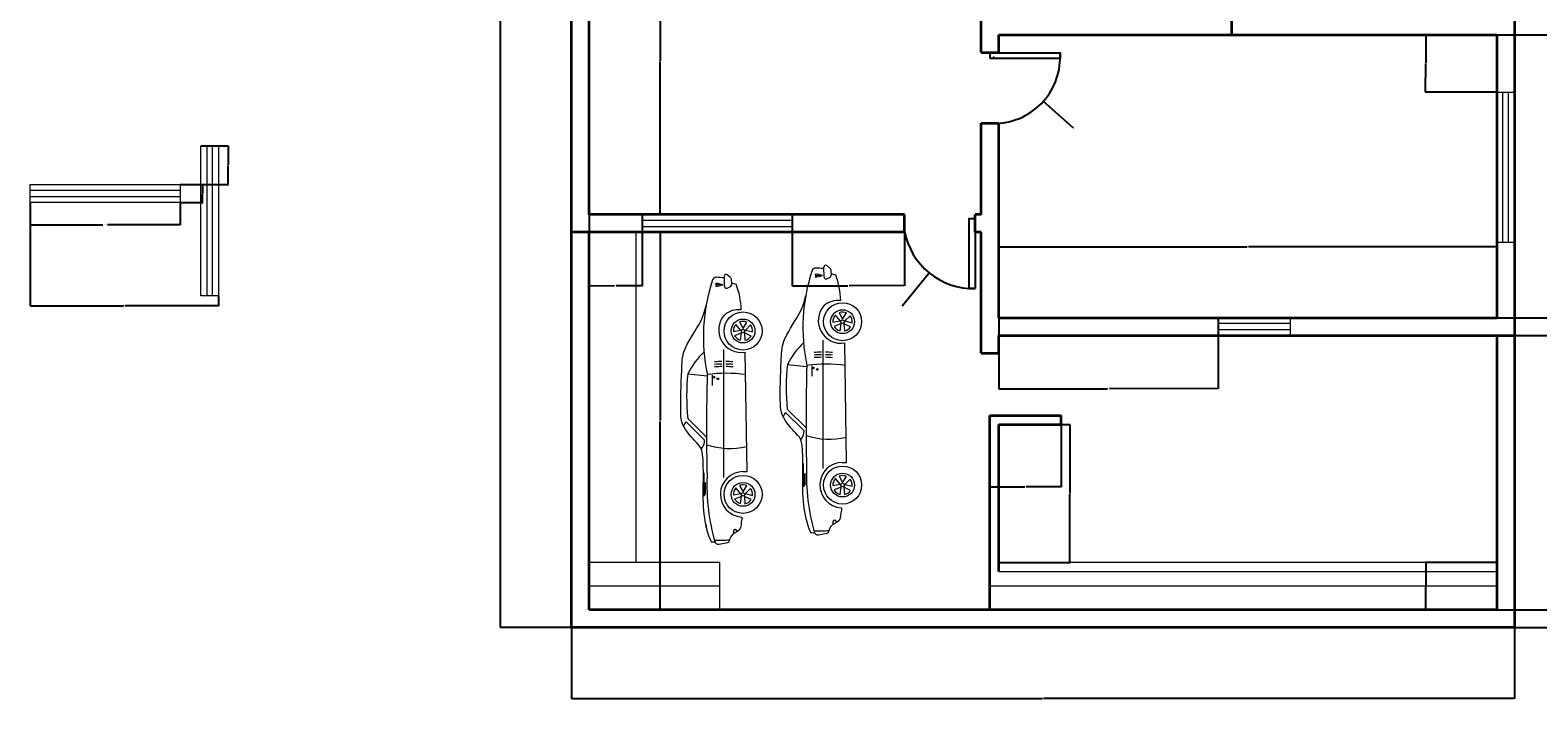
# Model space of a CAD drawing. Units: inches. Extents: x -52 to 1967, y 32 to 824.
# Tile 1 of 10: x -52 to 715, y 32 to 372. Entities that reach past the tile are written whole.
import ezdxf

# ---------------------------------------------------------------- set-up
doc = ezdxf.new("R2010")
doc.units = ezdxf.units.IN
for name, color, linetype, lineweight in [('A-ANNO-DIMS', 2, 'Continuous', 18), ('A-DOOR', 3, 'Continuous', 25), ('A-FLOR', 7, 'Continuous', 18), ('A-GLAZ', 4, 'Continuous', 18), ('A-SITE-VEHI', 8, 'Continuous', 13), ('A-WALL', 7, 'Continuous', 35)]:
    doc.layers.add(name, color=color, linetype=linetype, lineweight=lineweight)
doc.styles.get("Standard").update_dxf_attribs({"font": 'arial.ttf'})
doc.dimstyles.get("Standard").update_dxf_attribs({"dimtxt": 0.18, "dimasz": 0.18, "dimexe": 0.18, "dimexo": 0.0625, "dimgap": 0.09, "dimtad": 0, "dimtih": 1, "dimtoh": 1, "dimdec": 4, "dimzin": 0, "dimdsep": 46, "dimtxsty": 'Standard', "dimcen": 0.09, "dimadec": 0, "dimazin": 0, "dimtfac": 1, "dimtdec": 4, "dimtofl": 0, "dimtmove": 0, "dimatfit": 3, "dimfxl": 1, "dimtolj": 1, "dimtzin": 0, "dimarcsym": 0})

# ---------------------------------------------------------------- blocks, each defined once
blk = doc.blocks.new('*U16')
for p, q in [((72.9, 40.2), (85.8, 53.2)), ((75, 38.8), (88.1, 52)), ((119.4, 51.9), (117.9, 38.3)), ((50.1, 41.1), (34.3, 41)), ((43.3, 39.8), (35.2, 39.8)), ((35.3, 40.5), (50.1, 40.6)), ((111.1, 34.7), (118.5, 34.6)), ((46.7, 26.8), (136.3, 26.8)), ((179.3, 24.4), (180.3, 22.5)), ((180.4, 26.2), (187.5, 26.4)), ((182.6, 21.1), (184.9, 21.3)), ((186.7, 22.2), (188.5, 24.4)), ((7.4, 19.8), (9.7, 19.8)), ((9.8, 17.9), (8.5, 17.9)), ((10.4, 19.2), (10.4, 18.6)), ((50.9, 13.5), (50.9, 10.5))]:
    blk.add_line(p, q)
for points in [[(35.3, 39.9), (35.3, 40.3, 0.269532), (35.1, 40.5), (34.4, 41, 0.575383), (34.2, 40.8), (34.2, 40.5, 0.269532), (34.3, 40.2), (35.1, 39.8, 0.575383)], [(31.3, 7.7), (33.5, 12.4), (28.4, 12, 0.199906)], [(28.5, 15.1), (33.6, 14.4), (31.7, 19.2, 0.199906)], [(39.2, 8.1), (35.5, 11.7), (34.2, 6.7, 0.199906)], [(34.6, 20.1), (35.6, 15), (39.5, 18.3, 0.199906)], [(41.2, 15.7), (36.7, 13.3), (41.1, 10.6, 0.199906)], [(142.8, 15.1), (148, 14.4), (146, 19.2, 0.199906)], [(145.7, 7.7), (147.9, 12.4), (142.8, 12, 0.199906)], [(153.5, 8.1), (149.8, 11.7), (148.6, 6.7, 0.199906)], [(149, 20.1), (149.9, 15), (153.9, 18.3, 0.199906)], [(155.6, 15.7), (151.1, 13.3), (155.4, 10.6, 0.199906)]]:
    blk.add_lwpolyline(points, format="xyb", close=True)
for points in [[(181.6, 27.5), (181.5, 31.9), (180.5, 32.4)], [(181.6, 27.5), (181.5, 31.9), (182.6, 32.5)], [(50.9, 10.5), (134.4, 11.8)]]:
    blk.add_lwpolyline(points)
for centre, radius in [((35, 13.3), 13.3), ((35, 13.3), 8.35), ((115.9, 31), 0.619), ((149.3, 13.3), 13.3), ((149.3, 13.3), 8.35), ((35, 13.3), 1.25), ((149.3, 13.3), 1.25)]:
    blk.add_circle(centre, radius)
for centre, radius, start, end in [((114.6, 105.1), 59.4, 237.6103, 240.9785), ((103.5, -95), 147.8, 83.8163, 95.9705), ((73.3, 50.5), 10.3, 230.424, 268.0085), ((95.5, 3.9), 53.6, 43.2748, 63.5665), ((42.2, -111.3), 149.9, 87.8393, 105.8096), ((20.5, -3.2), 43.1, 98.5304, 116.112), ((79.2, 30.1), 76.3, 177.5773, 185.5205), ((80.1, -1364.1), 1403, 88.423, 91.3179), ((118.3, 22.5), 51.2, 161.4307, 193.2363), ((145.2, -84.9), 126, 71.5283, 102.1242), ((25.7, 24.9), 94, 351.8279, 8.1674), ((45.6, 26.8), 78.8, 0.852, 4.6556), ((47.4, 26.9), 78.8, 0.852, 4.6556), ((49.2, 26.9), 78.8, 0.852, 4.6556), ((216.3, 37.8), 36.2, 188.4683, 196.5315), ((146.7, 37), 36.2, 344.7432, 352.8063), ((184.3, 32.3), 2.49, 357.932, 71.5283), ((116.6, 34.7), 70.3, 353.1942, 357.932), ((35, 13.3), 15.9, 0.6373, 176.3412), ((45.6, 26.8), 78.8, 355.2644, 358.8633), ((47.4, 26.9), 78.8, 355.2644, 358.8633), ((49.2, 26.9), 78.8, 355.2644, 358.8633), ((150.1, 14.4), 15.9, 49.2263, 189.1528), ((149.4, 16.5), 14.8, 352.7285, 41.6613), ((180.4, 24.9), 1.25, 91.939, 207.109), ((182.5, 23.6), 2.49, 207.109, 273.4677), ((114.2, 37), 70.3, 344.3985, 346.9385), ((184.8, 23.8), 2.49, 273.4677, 320.1683), ((187.6, 25.2), 1.25, 320.1683, 91.939), ((9.7, 19.2), 0.623, 0.6373, 90.6373), ((9.8, 18.6), 0.623, 270.6373, 0.6373), ((162.5, 70.8), 56.2, 271.6865, 290.2774)]:
    blk.add_arc(centre, radius, start, end)
blk.add_ellipse((116.9, 33.6), major_axis=(-0.63, -0.007), ratio=0.610043)
for points, knots in [([(11.4, 38.9), (18.1, 40.2), (30.9, 42), (64.8, 40.1), (70.2, 44.9), (82.4, 56.4), (99.2, 57.3), (116.1, 56.4), (133, 55.9), (145.2, 49.9), (153.6, 43.8), (161.2, 40.7), (164.9, 39.7), (167.3, 39.2)], [18.629823, 18.629823, 18.629823, 18.629823, 19.527405, 20.700571, 21.107983, 21.608568, 21.92336, 23.151359, 23.716171, 23.908743, 24.77794, 24.943072, 25.187755, 25.187755, 25.187755, 25.187755]), ([(19.1, 14.4), (19, 14.2), (18.5, 13.8), (15.4, 15), (9.2, 13.9), (7.3, 22.2), (3, 22.7), (1.3, 23.6), (0.6, 26.9), (-1, 31.5), (1.5, 32.6), (1.5, 34.1), (1.5, 34.8), (1.5, 35.1), (1.5, 35.3), (1.6, 35.5)], [16.815853, 16.815853, 16.815853, 16.815853, 16.838212, 16.885395, 17.18439, 17.479846, 17.654423, 17.670693, 17.696923, 18.016358, 18.052739, 18.140805, 18.140805, 18.140805, 18.172382, 18.172382, 18.172382, 18.172382])]:
    blk.add_open_spline(points, degree=3, knots=knots)
blk = doc.blocks.new('WIN-WIDE-76IN')
for p, q in [((0, 0), (0, 9)), ((0, 9), (76.34, 9)), ((76.34, 9), (76.34, 0)), ((76.34, 6), (0, 6)), ((0, 3), (76.34, 3)), ((76.34, 0), (0, 0))]:
    blk.add_line(p, q)
blk = doc.blocks.new('WIN-NARROW-37IN')
for p, q in [((0, 0), (0, 9)), ((0, 9), (36.78, 9)), ((36.78, 0), (36.78, 9)), ((36.78, 6), (0, 6)), ((0, 3), (36.78, 3)), ((36.78, 0), (0, 0))]:
    blk.add_line(p, q)
blk = doc.blocks.new('DOOR-LEAF-36IN')
blk.add_lwpolyline([(0, 0), (-2.98, 0), (-2.98, 35.63), (0, 35.63)], close=True)
blk = doc.blocks.new('*D21')
at = {"layer": 'A-ANNO-DIMS', "color": 0, "lineweight": -2, "transparency": 16777216}
for p, q in [((-52.4, 284.15), (-52.4, 272.58)), ((23.94, 284.15), (23.94, 272.58)), ((-52.22, 272.76), (-15.35, 272.76)), ((23.76, 272.76), (-13.11, 272.76))]:
    blk.add_line(p, q, dxfattribs=at)
at = {"layer": 'A-ANNO-DIMS', "color": 0, "transparency": 16777216}
for points in [[(-52.22, 272.79), (-52.22, 272.73), (-52.4, 272.76)], [(23.76, 272.79), (23.76, 272.73), (23.94, 272.76)]]:
    blk.add_solid(points, dxfattribs=at)
at = {"layer": 'Defpoints', "color": 0, "transparency": 16777216}
for p in [(-52.4, 284.21), (23.94, 284.21), (23.94, 272.76)]:
    blk.add_point(p, dxfattribs=at)
at = {"layer": 'A-ANNO-DIMS', "color": 0, "transparency": 16777216, "insert": (-14.23, 272.76), "char_height": 0.18, "attachment_point": 5}
blk.add_mtext('\\A1;WINDOW 76 TYP.', dxfattribs=at)
blk = doc.blocks.new('*D22')
at = {"layer": 'A-ANNO-DIMS', "color": 0, "lineweight": -2, "transparency": 16777216}
for p, q in [((24, 293.21), (35.57, 293.21)), ((35.39, 293.03), (35.39, 288.89)), ((24, 284.21), (35.57, 284.21)), ((35.39, 284.39), (35.39, 288.53))]:
    blk.add_line(p, q, dxfattribs=at)
at = {"layer": 'A-ANNO-DIMS', "color": 0, "transparency": 16777216}
for points in [[(35.36, 293.03), (35.42, 293.03), (35.39, 293.21)], [(35.36, 284.39), (35.42, 284.39), (35.39, 284.21)]]:
    blk.add_solid(points, dxfattribs=at)
at = {"layer": 'Defpoints', "color": 0, "transparency": 16777216}
for p in [(23.94, 293.21), (35.39, 293.21), (23.94, 284.21)]:
    blk.add_point(p, dxfattribs=at)
at = {"layer": 'A-ANNO-DIMS', "color": 0, "transparency": 16777216, "insert": (35.39, 288.71), "char_height": 0.18, "attachment_point": 5}
blk.add_mtext('\\A1;9 TYP.', dxfattribs=at)
blk = doc.blocks.new('*D53')
at = {"layer": 'A-ANNO-DIMS', "color": 0, "lineweight": -2, "transparency": 16777216}
for p, q in [((223.03, 67.91), (223.03, 31.66)), ((703.03, 67.91), (703.03, 31.66)), ((223.21, 31.84), (462.74, 31.84)), ((702.85, 31.84), (463.32, 31.84))]:
    blk.add_line(p, q, dxfattribs=at)
at = {"layer": 'A-ANNO-DIMS', "color": 0, "transparency": 16777216}
for points in [[(223.21, 31.87), (223.21, 31.81), (223.03, 31.84)], [(702.85, 31.87), (702.85, 31.81), (703.03, 31.84)]]:
    blk.add_solid(points, dxfattribs=at)
at = {"layer": 'Defpoints', "color": 0, "transparency": 16777216}
for p in [(223.03, 67.97), (703.03, 67.97), (703.03, 31.84)]:
    blk.add_point(p, dxfattribs=at)
at = {"layer": 'A-ANNO-DIMS', "color": 0, "transparency": 16777216, "insert": (463.03, 31.84), "char_height": 0.18, "attachment_point": 5}
blk.add_mtext('\\A1;480', dxfattribs=at)
blk = doc.blocks.new('*D54')
at = {"layer": 'A-ANNO-DIMS', "color": 0, "lineweight": -2, "transparency": 16777216}
for p, q in [((222.96, 787.97), (186.72, 787.97)), ((186.9, 787.79), (186.9, 428.16)), ((186.9, 68.15), (186.9, 427.79)), ((222.96, 67.97), (186.72, 67.97))]:
    blk.add_line(p, q, dxfattribs=at)
at = {"layer": 'A-ANNO-DIMS', "color": 0, "transparency": 16777216}
for points in [[(186.87, 787.79), (186.93, 787.79), (186.9, 787.97)], [(186.87, 68.15), (186.93, 68.15), (186.9, 67.97)]]:
    blk.add_solid(points, dxfattribs=at)
at = {"layer": 'Defpoints', "color": 0, "transparency": 16777216}
for p in [(186.9, 787.97), (223.03, 787.97), (223.03, 67.97)]:
    blk.add_point(p, dxfattribs=at)
at = {"layer": 'A-ANNO-DIMS', "color": 0, "transparency": 16777216, "insert": (186.9, 427.97), "char_height": 0.18, "attachment_point": 5}
blk.add_mtext('\\A1;720', dxfattribs=at)
blk = doc.blocks.new('*D60')
at = {"layer": 'A-ANNO-DIMS', "color": 0, "lineweight": -2, "transparency": 16777216}
for p, q in [((232.09, 433.97), (268.34, 433.97)), ((268.16, 433.79), (268.16, 356.16)), ((268.16, 278.15), (268.16, 355.79)), ((232.09, 277.97), (268.34, 277.97))]:
    blk.add_line(p, q, dxfattribs=at)
at = {"layer": 'A-ANNO-DIMS', "color": 0, "transparency": 16777216}
for points in [[(268.13, 433.79), (268.19, 433.79), (268.16, 433.97)], [(268.13, 278.15), (268.19, 278.15), (268.16, 277.97)]]:
    blk.add_solid(points, dxfattribs=at)
at = {"layer": 'Defpoints', "color": 0, "transparency": 16777216}
for p in [(232.03, 433.97), (232.03, 277.97), (268.16, 277.97)]:
    blk.add_point(p, dxfattribs=at)
at = {"layer": 'A-ANNO-DIMS', "color": 0, "transparency": 16777216, "insert": (268.16, 355.97), "char_height": 0.18, "attachment_point": 5}
blk.add_mtext('\\A1;156', dxfattribs=at)
blk = doc.blocks.new('*D61')
at = {"layer": 'A-ANNO-DIMS', "color": 0, "lineweight": -2, "transparency": 16777216}
for p, q in [((232.09, 268.97), (268.34, 268.97)), ((268.16, 268.79), (268.16, 173.16)), ((268.16, 77.15), (268.16, 172.79)), ((232.09, 76.97), (268.34, 76.97))]:
    blk.add_line(p, q, dxfattribs=at)
at = {"layer": 'A-ANNO-DIMS', "color": 0, "transparency": 16777216}
for points in [[(268.13, 268.79), (268.19, 268.79), (268.16, 268.97)], [(268.13, 77.15), (268.19, 77.15), (268.16, 76.97)]]:
    blk.add_solid(points, dxfattribs=at)
at = {"layer": 'Defpoints', "color": 0, "transparency": 16777216}
for p in [(232.03, 268.97), (232.03, 76.97), (268.16, 76.97)]:
    blk.add_point(p, dxfattribs=at)
at = {"layer": 'A-ANNO-DIMS', "color": 0, "transparency": 16777216, "insert": (268.16, 172.97), "char_height": 0.18, "attachment_point": 5}
blk.add_mtext('\\A1;192', dxfattribs=at)
blk = doc.blocks.new('*D62')
at = {"layer": 'A-ANNO-DIMS', "color": 0, "lineweight": -2, "transparency": 16777216}
for p, q in [((440.53, 225.54), (440.53, 261.78)), ((440.71, 261.6), (566.88, 261.6)), ((693.85, 261.6), (567.67, 261.6)), ((694.03, 225.54), (694.03, 261.78))]:
    blk.add_line(p, q, dxfattribs=at)
at = {"layer": 'A-ANNO-DIMS', "color": 0, "transparency": 16777216}
for points in [[(440.71, 261.63), (440.71, 261.57), (440.53, 261.6)], [(693.85, 261.63), (693.85, 261.57), (694.03, 261.6)]]:
    blk.add_solid(points, dxfattribs=at)
at = {"layer": 'Defpoints', "color": 0, "transparency": 16777216}
for p in [(694.03, 261.6), (440.53, 225.47), (694.03, 225.47)]:
    blk.add_point(p, dxfattribs=at)
at = {"layer": 'A-ANNO-DIMS', "color": 0, "transparency": 16777216, "insert": (567.28, 261.6), "char_height": 0.18, "attachment_point": 5}
blk.add_mtext('\\A1;253.5', dxfattribs=at)
blk = doc.blocks.new('*D67')
at = {"layer": 'A-ANNO-DIMS', "color": 0, "lineweight": -2, "transparency": 16777216}
for p, q in [((694.09, 369.47), (739.35, 369.47)), ((739.17, 369.29), (739.17, 297.65)), ((739.17, 225.65), (739.17, 297.29)), ((694.09, 225.47), (739.35, 225.47))]:
    blk.add_line(p, q, dxfattribs=at)
at = {"layer": 'A-ANNO-DIMS', "color": 0, "transparency": 16777216}
for points in [[(739.14, 369.29), (739.2, 369.29), (739.17, 369.47)], [(739.14, 225.65), (739.2, 225.65), (739.17, 225.47)]]:
    blk.add_solid(points, dxfattribs=at)
at = {"layer": 'Defpoints', "color": 0, "transparency": 16777216}
for p in [(694.03, 369.47), (739.17, 369.47), (694.03, 225.47)]:
    blk.add_point(p, dxfattribs=at)
at = {"layer": 'A-ANNO-DIMS', "color": 0, "transparency": 16777216, "insert": (739.17, 297.47), "char_height": 0.18, "attachment_point": 5}
blk.add_mtext('\\A1;144', dxfattribs=at)
blk = doc.blocks.new('*D68')
at = {"layer": 'A-ANNO-DIMS', "color": 0, "lineweight": -2, "transparency": 16777216}
for p, q in [((694.09, 216.47), (739.35, 216.47)), ((739.17, 216.29), (739.17, 146.91)), ((739.17, 77.15), (739.17, 146.54)), ((694.09, 76.97), (739.35, 76.97))]:
    blk.add_line(p, q, dxfattribs=at)
at = {"layer": 'A-ANNO-DIMS', "color": 0, "transparency": 16777216}
for points in [[(739.14, 216.29), (739.2, 216.29), (739.17, 216.47)], [(739.14, 77.15), (739.2, 77.15), (739.17, 76.97)]]:
    blk.add_solid(points, dxfattribs=at)
at = {"layer": 'Defpoints', "color": 0, "transparency": 16777216}
for p in [(694.03, 216.47), (739.17, 216.47), (694.03, 76.97)]:
    blk.add_point(p, dxfattribs=at)
at = {"layer": 'A-ANNO-DIMS', "color": 0, "transparency": 16777216, "insert": (739.17, 146.72), "char_height": 0.18, "attachment_point": 5}
blk.add_mtext('\\A1;139.5', dxfattribs=at)
blk = doc.blocks.new('*D69')
at = {"layer": 'A-ANNO-DIMS', "color": 0, "lineweight": -2, "transparency": 16777216}
for p, q in [((694.09, 76.97), (739.35, 76.97)), ((739.17, 76.79), (739.17, 72.66)), ((739.17, 68.15), (739.17, 72.29)), ((703.09, 67.97), (739.35, 67.97))]:
    blk.add_line(p, q, dxfattribs=at)
at = {"layer": 'A-ANNO-DIMS', "color": 0, "transparency": 16777216}
for points in [[(739.14, 76.79), (739.2, 76.79), (739.17, 76.97)], [(739.14, 68.15), (739.2, 68.15), (739.17, 67.97)]]:
    blk.add_solid(points, dxfattribs=at)
at = {"layer": 'Defpoints', "color": 0, "transparency": 16777216}
for p in [(694.03, 76.97), (739.17, 76.97), (703.03, 67.97)]:
    blk.add_point(p, dxfattribs=at)
at = {"layer": 'A-ANNO-DIMS', "color": 0, "transparency": 16777216, "insert": (739.17, 72.47), "char_height": 0.18, "attachment_point": 5}
blk.add_mtext('\\A1;9', dxfattribs=at)
blk = doc.blocks.new('*D73')
at = {"layer": 'A-ANNO-DIMS', "color": 0, "lineweight": -2, "transparency": 16777216}
for p, q in [((232.03, 277.91), (231.93, 241.66)), ((259.09, 277.84), (258.99, 241.59)), ((232.11, 241.84), (244.99, 241.81)), ((258.81, 241.77), (245.92, 241.8))]:
    blk.add_line(p, q, dxfattribs=at)
at = {"layer": 'A-ANNO-DIMS', "color": 0, "transparency": 16777216}
for points in [[(232.11, 241.87), (232.11, 241.81), (231.93, 241.84)], [(258.81, 241.8), (258.81, 241.74), (258.99, 241.77)]]:
    blk.add_solid(points, dxfattribs=at)
at = {"layer": 'Defpoints', "color": 0, "transparency": 16777216}
for p in [(232.03, 277.97), (259.09, 277.9), (231.93, 241.84)]:
    blk.add_point(p, dxfattribs=at)
at = {"layer": 'A-ANNO-DIMS', "color": 0, "transparency": 16777216, "insert": (245.46, 241.81), "char_height": 0.18, "attachment_point": 5}
blk.add_mtext('\\A1;27.065', dxfattribs=at)
blk = doc.blocks.new('*D74')
at = {"layer": 'A-ANNO-DIMS', "color": 0, "lineweight": -2, "transparency": 16777216}
for p, q in [((335.43, 277.84), (335.48, 241.59)), ((392.53, 277.91), (392.58, 241.66)), ((335.66, 241.77), (363.72, 241.81)), ((392.39, 241.84), (364.33, 241.81))]:
    blk.add_line(p, q, dxfattribs=at)
at = {"layer": 'A-ANNO-DIMS', "color": 0, "transparency": 16777216}
for points in [[(335.66, 241.8), (335.66, 241.74), (335.48, 241.77)], [(392.39, 241.87), (392.39, 241.81), (392.57, 241.84)]]:
    blk.add_solid(points, dxfattribs=at)
at = {"layer": 'Defpoints', "color": 0, "transparency": 16777216}
for p in [(335.43, 277.9), (392.53, 277.97), (335.48, 241.77)]:
    blk.add_point(p, dxfattribs=at)
at = {"layer": 'A-ANNO-DIMS', "color": 0, "transparency": 16777216, "insert": (364.03, 241.81), "char_height": 0.18, "attachment_point": 5}
blk.add_mtext('\\A1;57.1', dxfattribs=at)
blk = doc.blocks.new('*D79')
at = {"layer": 'A-ANNO-DIMS', "color": 0, "lineweight": -2, "transparency": 16777216}
for p, q in [((440.53, 225.41), (440.57, 189.16)), ((552.17, 225.54), (552.21, 189.29)), ((440.75, 189.34), (495.94, 189.41)), ((552.03, 189.47), (496.85, 189.41))]:
    blk.add_line(p, q, dxfattribs=at)
at = {"layer": 'A-ANNO-DIMS', "color": 0, "transparency": 16777216}
for points in [[(440.75, 189.37), (440.75, 189.31), (440.57, 189.34)], [(552.03, 189.5), (552.03, 189.44), (552.21, 189.47)]]:
    blk.add_solid(points, dxfattribs=at)
at = {"layer": 'Defpoints', "color": 0, "transparency": 16777216}
for p in [(440.53, 225.47), (552.17, 225.6), (440.57, 189.34)]:
    blk.add_point(p, dxfattribs=at)
at = {"layer": 'A-ANNO-DIMS', "color": 0, "transparency": 16777216, "insert": (496.39, 189.41), "char_height": 0.18, "attachment_point": 5}
blk.add_mtext('\\A1;111.65', dxfattribs=at)
blk = doc.blocks.new('*D85')
at = {"layer": 'A-ANNO-DIMS', "color": 0, "lineweight": -2, "transparency": 16777216}
for p, q in [((693.96, 369.47), (657.72, 369.61)), ((657.9, 369.43), (657.84, 355.14)), ((657.79, 340.49), (657.84, 354.78)), ((693.86, 340.18), (657.61, 340.31))]:
    blk.add_line(p, q, dxfattribs=at)
at = {"layer": 'A-ANNO-DIMS', "color": 0, "transparency": 16777216}
for points in [[(657.87, 369.43), (657.93, 369.43), (657.9, 369.61)], [(657.76, 340.49), (657.82, 340.49), (657.79, 340.31)]]:
    blk.add_solid(points, dxfattribs=at)
at = {"layer": 'Defpoints', "color": 0, "transparency": 16777216}
for p in [(657.9, 369.61), (694.03, 369.47), (693.92, 340.18)]:
    blk.add_point(p, dxfattribs=at)
at = {"layer": 'A-ANNO-DIMS', "color": 0, "transparency": 16777216, "insert": (657.84, 354.96), "char_height": 0.18, "attachment_point": 5}
blk.add_mtext('\\A1;29.296', dxfattribs=at)
blk = doc.blocks.new('*D90')
at = {"layer": 'A-ANNO-DIMS', "color": 0, "lineweight": -2, "transparency": 16777216}
for p, q in [((436.03, 175.65), (436.03, 139.4)), ((472.29, 175.65), (472.29, 139.4)), ((436.21, 139.58), (453.76, 139.58)), ((472.11, 139.58), (454.55, 139.58))]:
    blk.add_line(p, q, dxfattribs=at)
at = {"layer": 'A-ANNO-DIMS', "color": 0, "transparency": 16777216}
for points in [[(436.21, 139.61), (436.21, 139.55), (436.03, 139.58)], [(472.11, 139.61), (472.11, 139.55), (472.29, 139.58)]]:
    blk.add_solid(points, dxfattribs=at)
at = {"layer": 'Defpoints', "color": 0, "transparency": 16777216}
for p in [(436.03, 175.71), (472.29, 175.71), (436.03, 139.58)]:
    blk.add_point(p, dxfattribs=at)
at = {"layer": 'A-ANNO-DIMS', "color": 0, "transparency": 16777216, "insert": (454.16, 139.58), "char_height": 0.18, "attachment_point": 5}
blk.add_mtext('\\A1;36.26', dxfattribs=at)
blk = doc.blocks.new('*D91')
at = {"layer": 'A-ANNO-DIMS', "color": 0, "lineweight": -2, "transparency": 16777216}
for p, q in [((440.59, 171.21), (476.84, 171.21)), ((476.66, 171.03), (476.66, 136.27)), ((476.66, 101.15), (476.66, 135.91)), ((440.59, 100.97), (476.84, 100.97))]:
    blk.add_line(p, q, dxfattribs=at)
at = {"layer": 'A-ANNO-DIMS', "color": 0, "transparency": 16777216}
for points in [[(476.63, 171.03), (476.69, 171.03), (476.66, 171.21)], [(476.63, 101.15), (476.69, 101.15), (476.66, 100.97)]]:
    blk.add_solid(points, dxfattribs=at)
at = {"layer": 'Defpoints', "color": 0, "transparency": 16777216}
for p in [(440.53, 171.21), (440.53, 100.97), (476.66, 100.97)]:
    blk.add_point(p, dxfattribs=at)
at = {"layer": 'A-ANNO-DIMS', "color": 0, "transparency": 16777216, "insert": (476.66, 136.09), "char_height": 0.18, "attachment_point": 5}
blk.add_mtext('\\A1;70.24', dxfattribs=at)
blk = doc.blocks.new('*D92')
at = {"layer": 'A-ANNO-DIMS', "color": 0, "lineweight": -2, "transparency": 16777216}
for p, q in [((693.96, 100.97), (657.72, 100.97)), ((657.9, 100.79), (657.9, 89.15)), ((657.9, 77.15), (657.9, 88.79)), ((693.96, 76.97), (657.72, 76.97))]:
    blk.add_line(p, q, dxfattribs=at)
at = {"layer": 'A-ANNO-DIMS', "color": 0, "transparency": 16777216}
for points in [[(657.87, 100.79), (657.93, 100.79), (657.9, 100.97)], [(657.87, 77.15), (657.93, 77.15), (657.9, 76.97)]]:
    blk.add_solid(points, dxfattribs=at)
at = {"layer": 'Defpoints', "color": 0, "transparency": 16777216}
for p in [(657.9, 100.97), (694.03, 100.97), (694.03, 76.97)]:
    blk.add_point(p, dxfattribs=at)
at = {"layer": 'A-ANNO-DIMS', "color": 0, "transparency": 16777216, "insert": (657.9, 88.97), "char_height": 0.18, "attachment_point": 5}
blk.add_mtext('\\A1;24', dxfattribs=at)
blk = doc.blocks.new('*D120')
at = {"layer": 'A-ANNO-DIMS', "color": 0, "lineweight": -2, "transparency": 16777216}
for p, q in [((-52.4, 284.15), (-52.4, 231.47)), ((-52.22, 231.65), (-4.85, 231.65)), ((43.31, 231.65), (-4.06, 231.65)), ((43.49, 236.53), (43.49, 231.47))]:
    blk.add_line(p, q, dxfattribs=at)
at = {"layer": 'A-ANNO-DIMS', "color": 0, "transparency": 16777216}
for points in [[(-52.22, 231.68), (-52.22, 231.62), (-52.4, 231.65)], [(43.31, 231.68), (43.31, 231.62), (43.49, 231.65)]]:
    blk.add_solid(points, dxfattribs=at)
at = {"layer": 'Defpoints', "color": 0, "transparency": 16777216}
for p in [(-52.4, 284.21), (43.49, 236.6), (43.49, 231.65)]:
    blk.add_point(p, dxfattribs=at)
at = {"layer": 'A-ANNO-DIMS', "color": 0, "transparency": 16777216, "insert": (-4.46, 231.65), "char_height": 0.18, "attachment_point": 5}
blk.add_mtext('\\A1;95.88', dxfattribs=at)
blk = doc.blocks.new('*D121')
at = {"layer": 'A-ANNO-DIMS', "color": 0, "lineweight": -2, "transparency": 16777216}
for p, q in [((34.55, 312.94), (48.62, 312.94)), ((48.44, 312.76), (48.44, 303.26)), ((48.44, 293.39), (48.44, 302.89)), ((24, 293.21), (48.62, 293.21))]:
    blk.add_line(p, q, dxfattribs=at)
at = {"layer": 'A-ANNO-DIMS', "color": 0, "transparency": 16777216}
for points in [[(48.41, 312.76), (48.47, 312.76), (48.44, 312.94)], [(48.41, 293.39), (48.47, 293.39), (48.44, 293.21)]]:
    blk.add_solid(points, dxfattribs=at)
at = {"layer": 'Defpoints', "color": 0, "transparency": 16777216}
for p in [(34.49, 312.94), (23.94, 293.21), (48.44, 293.21)]:
    blk.add_point(p, dxfattribs=at)
at = {"layer": 'A-ANNO-DIMS', "color": 0, "transparency": 16777216, "insert": (48.44, 303.07), "char_height": 0.18, "attachment_point": 5}
blk.add_mtext('\\A1;19.724', dxfattribs=at)
blk = doc.blocks.new('*D136')
at = {"layer": 'A-ANNO-DIMS', "color": 0, "lineweight": -2, "transparency": 16777216}
for p, q in [((427.79, 276.08), (427.79, 276.26)), ((427.7, 276.17), (427.88, 276.17)), ((391.56, 231.69), (405.03, 248.23)), ((391.38, 231.69), (391.56, 231.69))]:
    blk.add_line(p, q, dxfattribs=at)
at = {"layer": 'A-ANNO-DIMS', "color": 0, "transparency": 16777216}
blk.add_solid([(405.01, 248.25), (405.06, 248.21), (405.15, 248.37)], dxfattribs=at)
at = {"layer": 'Defpoints', "color": 0, "transparency": 16777216}
for p in [(427.79, 276.17), (405.15, 248.37)]:
    blk.add_point(p, dxfattribs=at)
at = {"layer": 'A-ANNO-DIMS', "color": 0, "transparency": 16777216, "insert": (390.83, 231.69), "char_height": 0.18, "attachment_point": 5}
blk.add_mtext('\\A1;R35.854', dxfattribs=at)
blk = doc.blocks.new('*D140')
at = {"layer": 'A-ANNO-DIMS', "color": 0, "lineweight": -2, "transparency": 16777216}
for p, q in [((437.91, 358.13), (438.09, 358.13)), ((438, 358.04), (438, 358.22)), ((478.37, 322.13), (463.37, 335.51)), ((478.55, 322.13), (478.37, 322.13))]:
    blk.add_line(p, q, dxfattribs=at)
at = {"layer": 'A-ANNO-DIMS', "color": 0, "transparency": 16777216}
blk.add_solid([(463.39, 335.53), (463.35, 335.49), (463.23, 335.63)], dxfattribs=at)
at = {"layer": 'Defpoints', "color": 0, "transparency": 16777216}
for p in [(438, 358.13), (463.23, 335.63)]:
    blk.add_point(p, dxfattribs=at)
at = {"layer": 'A-ANNO-DIMS', "color": 0, "transparency": 16777216, "insert": (479.1, 322.13), "char_height": 0.18, "attachment_point": 5}
blk.add_mtext('\\A1;R33.806', dxfattribs=at)

msp = doc.modelspace()

# ---------------------------------------------------------------- linework, layer by layer
at = {"layer": 'A-DOOR'}
for centre, radius, start, end in [((438.0039, 358.1286), 33.8058, 272.7480387, 3.8021122), ((427.7931, 276.1667), 35.8539, 190.4950029, 271.1640797)]:
    msp.add_arc(centre, radius, start, end, dxfattribs=at)
at = {"layer": 'A-FLOR'}
for p, q in [((256.0273, 100.9731), (256.0273, 268.9731)), ((298.55, 100.9731), (232.0273, 100.9731)), ((298.55, 76.9731), (298.55, 100.9731)), ((694.0273, 100.9731), (440.5273, 100.9731)), ((440.5273, 96.4731), (694.0273, 96.4731)), ((298.55, 88.9731), (232.0273, 88.9731)), ((694.0273, 88.9731), (436.0273, 88.9731))]:
    msp.add_line(p, q, dxfattribs=at)
at = {"layer": 'A-WALL'}
for p, q in [((223.0273, 67.9731), (223.0273, 787.9731)), ((703.0273, 787.9731), (703.0273, 67.9731)), ((559.0273, 493.9731), (559.0273, 369.4731)), ((431.5273, 360.4731), (431.5273, 481.9731)), ((232.0273, 277.9731), (232.0273, 433.9731)), ((440.5273, 369.4731), (694.0273, 369.4731)), ((440.5273, 360.4731), (440.5273, 369.4731)), ((694.0273, 369.4731), (694.0273, 225.4731)), ((431.5273, 360.4731), (440.5273, 360.4731)), ((431.5273, 277.9731), (431.5273, 324.4731)), ((431.5273, 324.4731), (440.5273, 324.4731)), ((440.5273, 225.4731), (440.5273, 324.4731)), ((392.5273, 277.9731), (232.0273, 277.9731)), ((392.5273, 268.9731), (392.5273, 277.9731)), ((431.5273, 277.9731), (428.5273, 277.9731)), ((428.5273, 268.9731), (428.5273, 277.9731)), ((392.5273, 268.9731), (223.0273, 268.9731)), ((232.0273, 76.9731), (232.0273, 268.9731)), ((431.5273, 268.9731), (428.5273, 268.9731)), ((431.5273, 207.4731), (431.5273, 268.9731)), ((440.5273, 225.4731), (694.0273, 225.4731)), ((431.5273, 207.4731), (431.5273, 216.4731)), ((440.5273, 216.4731), (703.0273, 216.4731)), ((440.5273, 207.4731), (440.5273, 216.4731)), ((694.0273, 216.4731), (694.0273, 76.9731)), ((431.5273, 207.4731), (440.5273, 207.4731)), ((436.0273, 76.9731), (436.0273, 175.7124)), ((436.0273, 175.7124), (472.288, 175.7124)), ((440.5273, 96.4731), (440.5273, 171.2124)), ((440.5273, 171.2124), (472.288, 171.2124)), ((472.288, 171.2124), (472.288, 175.7124)), ((694.0273, 76.9731), (232.0273, 76.9731)), ((703.0273, 67.9731), (223.0273, 67.9731))]:
    msp.add_line(p, q, dxfattribs=at)

# ---------------------------------------------------------------- block references
at = {"layer": 'A-DOOR', "rotation": 269.9999999999999}
msp.add_blockref('DOOR-LEAF-36IN', (436.1893, 357.3563), dxfattribs=at)
at = {"layer": 'A-DOOR'}
msp.add_blockref('DOOR-LEAF-36IN', (428.5249, 240.3544), dxfattribs=at)
at = {"layer": 'A-GLAZ'}
for p, rotation in [((693.9176, 340.1773), 269.9999999999998), ((34.4864, 312.9352), 270)]:
    msp.add_blockref('WIN-WIDE-76IN', p, dxfattribs=dict(at, rotation=rotation))
for name, p in [('WIN-WIDE-76IN', (-52.398, 284.2112)), ('WIN-WIDE-76IN', (259.0918, 268.8979)), ('WIN-NARROW-37IN', (552.1728, 216.5994))]:
    msp.add_blockref(name, p, dxfattribs=at)
at = {"layer": 'A-SITE-VEHI', "xscale": 0.7270548335690084, "yscale": 0.7270548335690084, "zscale": 0.7270548335690084, "rotation": 90}
for p in [(320.0828, 110.222), (370.7342, 114.9528)]:
    msp.add_blockref('*U16', p, dxfattribs=at)

# ---------------------------------------------------------------- dimensions: what is measured, and where the dimension line sits
at = {"layer": 'A-ANNO-DIMS'}
for base, p1, p2, angle, override, picture, middle in [((186.8973, 787.9731), (223.0273, 67.9731), (223.0273, 787.9731), 90, {"dimdec": 0, "dimlfac": 1, "dimrnd": 0, "dimzin": 0, "dimdsep": 46, "dimlunit": 2}, '*D54', (186.8973, 427.9731)), ((268.1573, 277.9731), (232.0273, 433.9731), (232.0273, 277.9731), 270, {"dimdec": 0, "dimlfac": 1, "dimrnd": 0, "dimzin": 0, "dimdsep": 46, "dimlunit": 2}, '*D60', (268.1573, 355.9731)), ((657.8975, 369.6083), (693.9176, 340.1773), (694.0273, 369.4731), 89.7856057, {"dimdec": 3, "dimlfac": 1, "dimrnd": 0, "dimzin": 0, "dimdsep": 46, "dimlunit": 2}, '*D85', (657.8427, 354.9604)), ((739.1728, 369.4731), (694.0273, 225.4731), (694.0273, 369.4731), 90, {"dimdec": 0, "dimlfac": 1, "dimrnd": 0, "dimzin": 0, "dimdsep": 46, "dimlunit": 2}, '*D67', (739.1728, 297.4731)), ((48.4364, 293.2112), (34.4864, 312.9352), (23.9422, 293.2112), 90, {"dimdec": 3, "dimlfac": 1, "dimrnd": 0, "dimzin": 0, "dimdsep": 46, "dimlunit": 2}, '*D121', (48.4364, 303.0732)), ((231.9268, 241.8433), (259.0918, 277.8979), (232.0273, 277.9731), 179.8406149, {"dimdec": 3, "dimlfac": 1, "dimrnd": 0, "dimzin": 0, "dimdsep": 46, "dimlunit": 2}, '*D73', (245.459, 241.8056)), ((335.4796, 241.7679), (392.5273, 277.9731), (335.4319, 277.8979), 180.0755524, {"dimdec": 1, "dimlfac": 1, "dimrnd": 0, "dimzin": 0, "dimdsep": 46, "dimlunit": 2}, '*D74', (364.0272, 241.8055)), ((268.1573, 76.9731), (232.0273, 268.9731), (232.0273, 76.9731), 270, {"dimdec": 0, "dimlfac": 1, "dimrnd": 0, "dimzin": 0, "dimdsep": 46, "dimlunit": 2}, '*D61', (268.1573, 172.9731)), ((440.5681, 189.3432), (552.1728, 225.5994), (440.5273, 225.4731), 180.0648152, {"dimdec": 2, "dimlfac": 1, "dimrnd": 0, "dimzin": 0, "dimdsep": 46, "dimlunit": 2}, '*D79', (496.3909, 189.4063)), ((739.1728, 216.4731), (694.0273, 76.9731), (694.0273, 216.4731), 90, {"dimdec": 1, "dimlfac": 1, "dimrnd": 0, "dimzin": 0, "dimdsep": 46, "dimlunit": 2}, '*D68', (739.1728, 146.7231)), ((436.0273, 139.5824), (472.288, 175.7124), (436.0273, 175.7124), 180, {"dimdec": 2, "dimlfac": 1, "dimrnd": 0, "dimzin": 0, "dimdsep": 46, "dimlunit": 2}, '*D90', (454.1576, 139.5824)), ((476.6573, 100.9731), (440.5273, 171.2124), (440.5273, 100.9731), 270, {"dimdec": 2, "dimlfac": 1, "dimrnd": 0, "dimzin": 0, "dimdsep": 46, "dimlunit": 2}, '*D91', (476.6573, 136.0928)), ((657.8973, 100.9731), (694.0273, 76.9731), (694.0273, 100.9731), 90, {"dimdec": 0, "dimlfac": 1, "dimrnd": 0, "dimzin": 0, "dimdsep": 46, "dimlunit": 2}, '*D92', (657.8973, 88.9731)), ((739.1728, 76.9731), (703.0273, 67.9731), (694.0273, 76.9731), 90, {"dimdec": 0, "dimlfac": 1, "dimrnd": 0, "dimzin": 0, "dimdsep": 46, "dimlunit": 2}, '*D69', (739.1728, 72.4731))]:
    dim = msp.add_linear_dim(base=base, p1=p1, p2=p2, angle=angle, dimstyle='Standard', override=override, dxfattribs=at)
    dim.commit()
    dim.dimension.update_dxf_attribs({"geometry": picture, "text_midpoint": middle})
for center, mpoint, picture, middle in [((438.0039, 358.1286), (463.2349, 335.6291), '*D140', (479.1032, 322.1294)), ((427.7931, 276.1667), (405.147, 248.37), '*D136', (390.8299, 231.6919))]:
    dim = msp.add_radius_dim(center=center, mpoint=mpoint, dimstyle='Standard', override={"dimdec": 3, "dimlfac": 1, "dimrnd": 0, "dimzin": 0, "dimdsep": 46, "dimlunit": 2}, dxfattribs=at)
    dim.commit()
    dim.dimension.update_dxf_attribs({"geometry": picture, "text_midpoint": middle, "dimtype": 164})
dim = msp.add_linear_dim(base=(35.3932, 293.2112), p1=(23.9422, 284.2112), p2=(23.9422, 293.2112), angle=90, text='<> TYP.', dimstyle='Standard', override={"dimdec": 0, "dimlfac": 1, "dimrnd": 0, "dimzin": 0, "dimdsep": 46, "dimlunit": 2}, dxfattribs=at)
dim.commit()
dim.dimension.update_dxf_attribs({"geometry": '*D22', "text_midpoint": (35.3932, 288.7112)})
dim = msp.add_linear_dim(base=(23.9422, 272.7602), p1=(-52.398, 284.2112), p2=(23.9422, 284.2112), text='WINDOW <> TYP.', dimstyle='Standard', override={"dimdec": 0, "dimlfac": 1, "dimrnd": 0, "dimzin": 0, "dimdsep": 46, "dimlunit": 2}, dxfattribs=at)
dim.commit()
dim.dimension.update_dxf_attribs({"geometry": '*D21', "text_midpoint": (-14.2279, 272.7602)})
for base, p1, p2, override, picture, middle in [((43.4864, 231.645), (-52.398, 284.2112), (43.4864, 236.595), {"dimdec": 2, "dimlfac": 1, "dimrnd": 0, "dimzin": 0, "dimdsep": 46, "dimlunit": 2}, '*D120', (-4.4558, 231.645)), ((694.0273, 261.6031), (440.5273, 225.4731), (694.0273, 225.4731), {"dimdec": 1, "dimlfac": 1, "dimrnd": 0, "dimzin": 0, "dimdsep": 46, "dimlunit": 2}, '*D62', (567.2773, 261.6031)), ((703.0273, 31.8431), (223.0273, 67.9731), (703.0273, 67.9731), {"dimdec": 0, "dimlfac": 1, "dimrnd": 0, "dimzin": 0, "dimdsep": 46, "dimlunit": 2}, '*D53', (463.0273, 31.8431))]:
    dim = msp.add_linear_dim(base=base, p1=p1, p2=p2, dimstyle='Standard', override=override, dxfattribs=at)
    dim.commit()
    dim.dimension.update_dxf_attribs({"geometry": picture, "text_midpoint": middle})

doc.saveas('drawing.dxf')
